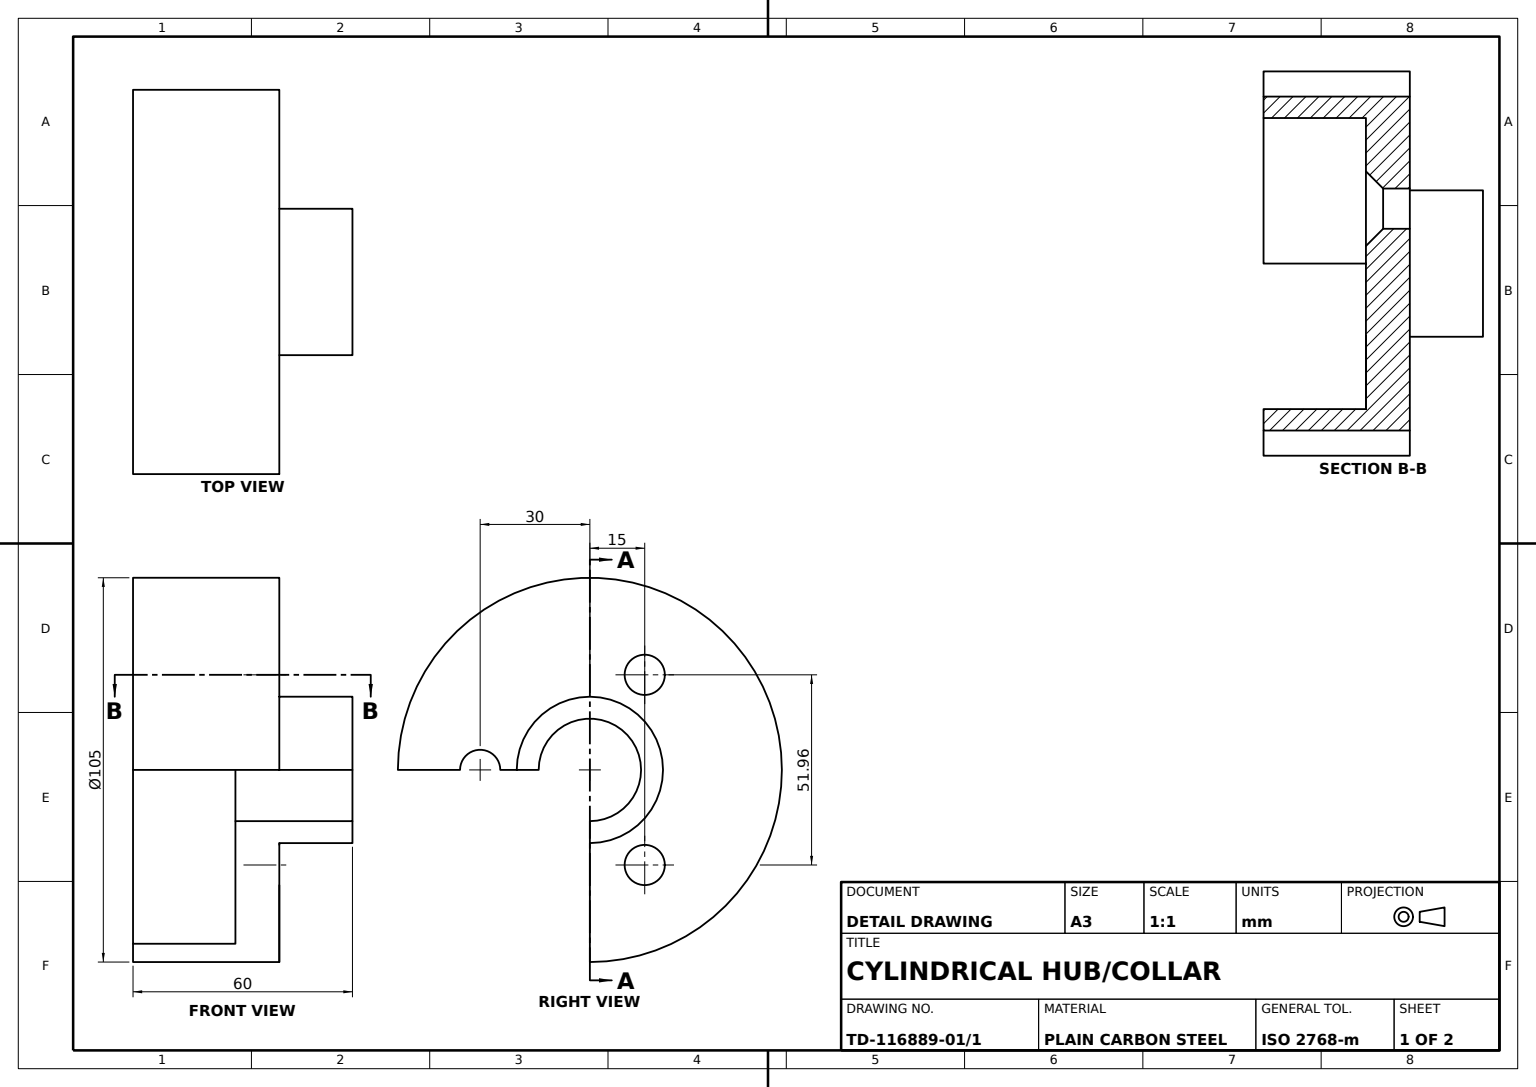
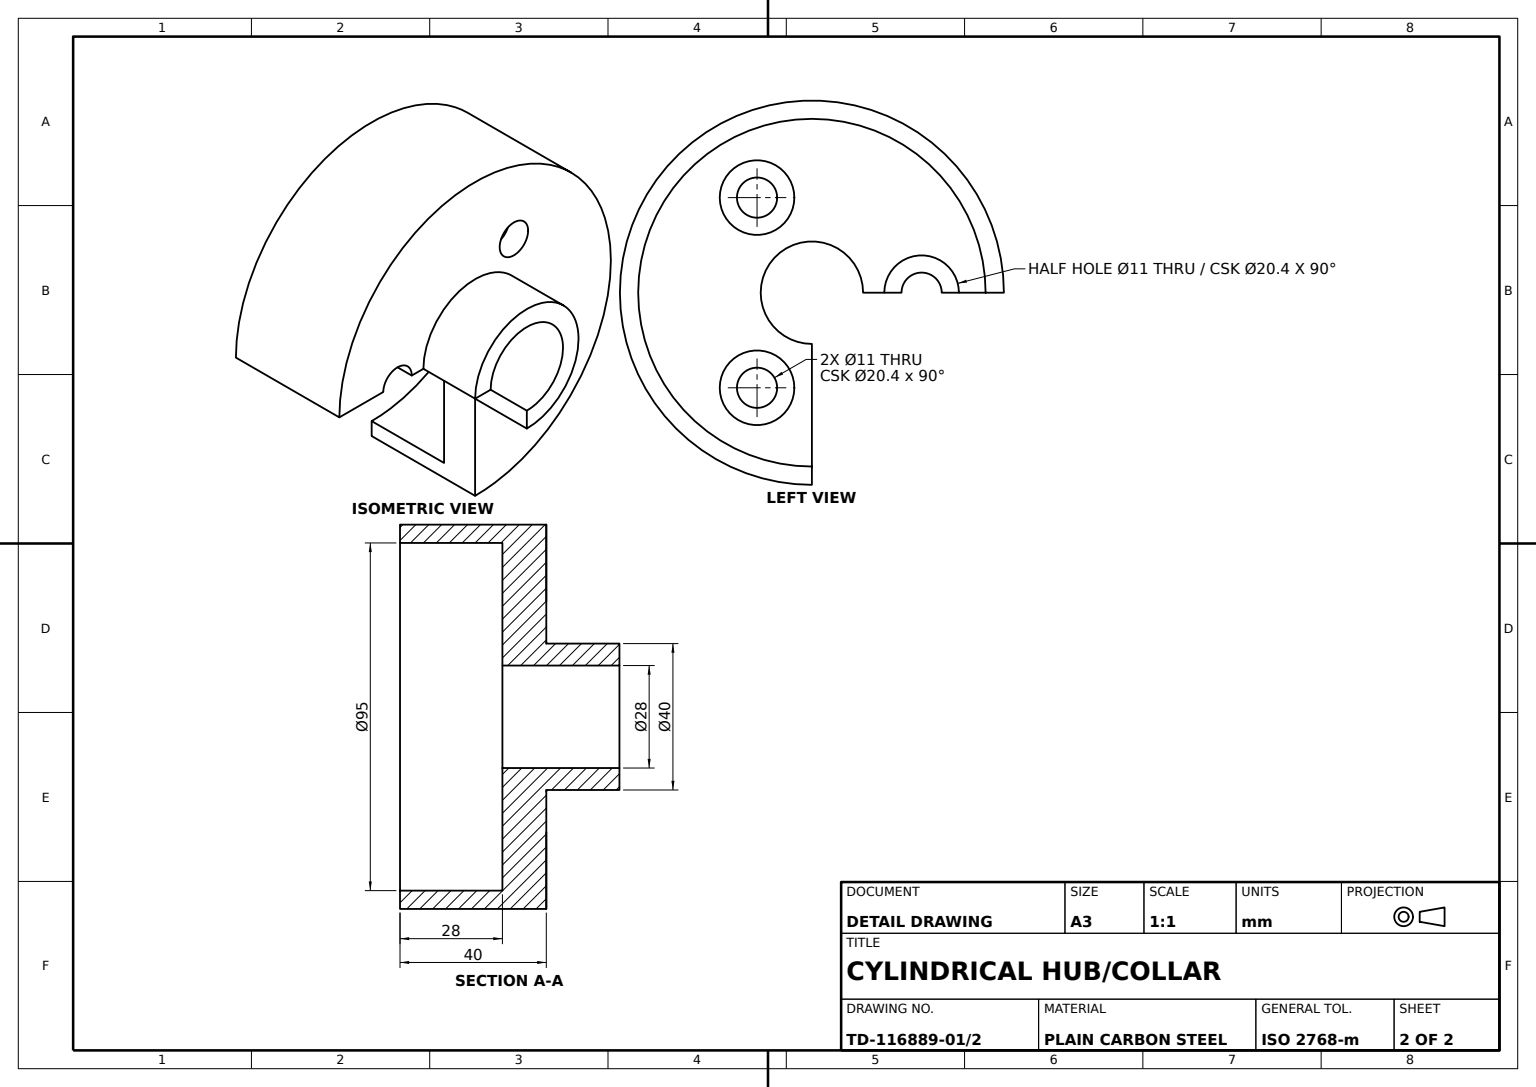
from build123d import *

# Parameters (mm, degrees)
COUNTERSUNK_HOLE_11_D             = 11
COUNTERSUNK_HOLE_11_CSINK_D       = 20.4
COUNTERSUNK_HOLE_11_CSINK_ANGLE   = 90
COUNTERSUNK_HOLE_PATTERN_3X_COUNT = 3
SIDE_SLOT_CUT_DEPTH               = 81.848623983
SIDE_SLOT_CUT_DEPTH_BACK          = 81.848623983


with BuildPart() as part:
    # Bed Profile Sketch → Bed Body Revolve (revolve)
    with BuildSketch(Plane(origin=(0, 0, 0), x_dir=(0, 0, -1), z_dir=(1, 0, 0))):
        Polygon((14, 30.393677345), (14, -1.606322655), (47.5, -1.606322655), (47.5, -29.606322655), (52.5, -29.606322655), (52.5, 10.393677345), (20, 10.393677345), (20, 30.393677345), align=None)
    revolve(axis=Axis((0, 0, 0), (0, 1, 0)))

    # Countersunk Hole Ø11 (through all)
    with Locations(Plane(origin=(0, -1.606322655, 30), x_dir=(0, 0, -1), z_dir=(0, -1, 0))):
        with Locations((0, 0)):
            countersunk_hole_11 = CounterSinkHole(COUNTERSUNK_HOLE_11_D / 2, COUNTERSUNK_HOLE_11_CSINK_D / 2, counter_sink_angle=COUNTERSUNK_HOLE_11_CSINK_ANGLE)

    # Countersunk Hole Pattern 3x: Countersunk Hole Ø11 ×3 about axis
    countersunk_hole_pattern_3x_axis = Axis((0, 0, 0), (0, 1, 0))
    for i in range(1, COUNTERSUNK_HOLE_PATTERN_3X_COUNT):
        add(countersunk_hole_11.rotate(countersunk_hole_pattern_3x_axis, i * 360 / COUNTERSUNK_HOLE_PATTERN_3X_COUNT), mode=Mode.SUBTRACT)

    # Side Slot Sketch → Side Slot Cut (cut, two sides: drawn at the far end of the back side and taken through both)
    with BuildSketch(Plane.XZ.offset(1.606322655).offset(-SIDE_SLOT_CUT_DEPTH_BACK)):
        with BuildLine():
            Line((0, 66.315052509), (0, 0))
            Line((0, 0), (70.372177226, 0))
            ThreePointArc((70.372177226, 0), (52.403266899, 51.428043669), (0, 66.315052509))
        make_face()
    extrude(amount=SIDE_SLOT_CUT_DEPTH + SIDE_SLOT_CUT_DEPTH_BACK, mode=Mode.SUBTRACT)


solid = part.part
